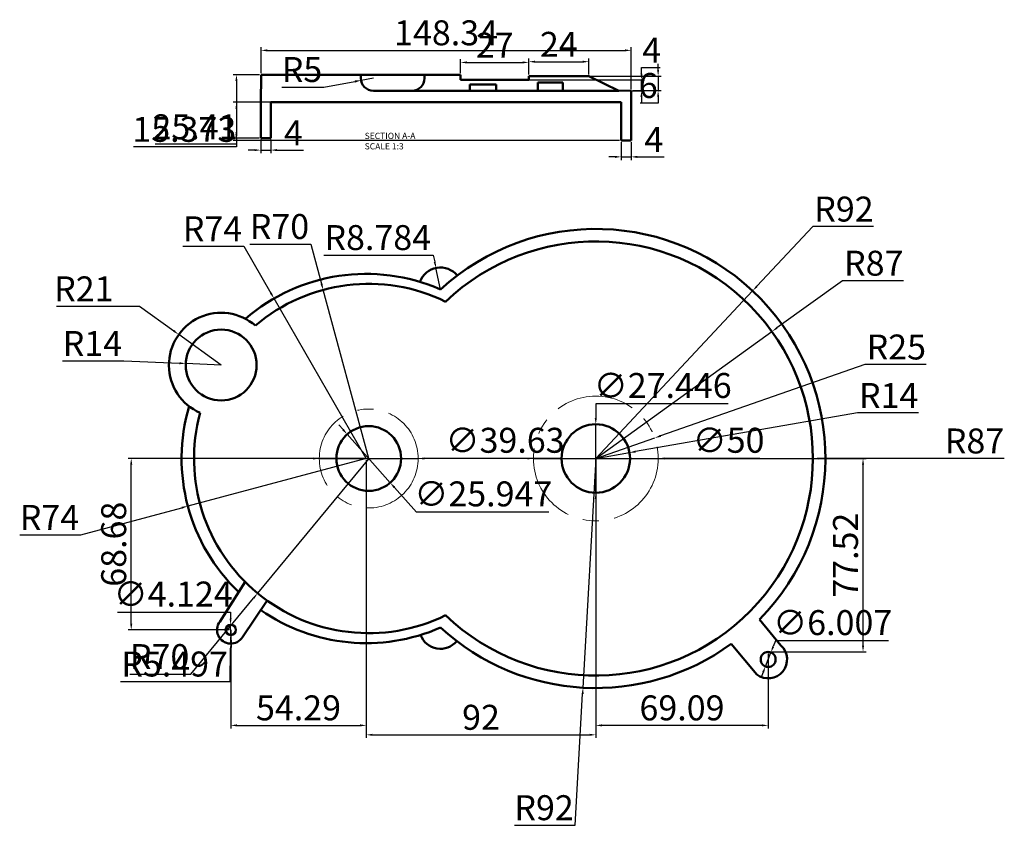
# Model space of a CAD drawing. Units: millimetres. Extents: x 828 to 2987, y 979 to 1807.
# Tile 3 of 6: x 828 to 1223, y 1483 to 1807. Entities that reach past the tile are written whole.
import ezdxf

# ---------------------------------------------------------------- set-up
doc = ezdxf.new("R2010")
doc.units = ezdxf.units.MM
doc.linetypes.add('CENTER', pattern=[50.8, 31.75, -6.35, 6.35, -6.35])
for name, color, linetype, lineweight in [('M-CNTR', 1, 'CENTER', 18), ('M-DIMS', 2, 'Continuous', 25), ('M-OUTL', 7, 'Continuous', 50), ('M-TEXT', 3, 'Continuous', 25)]:
    doc.layers.add(name, color=color, linetype=linetype, lineweight=lineweight)
doc.styles.get("Standard").update_dxf_attribs({"font": 'arial.ttf'})
doc.dimstyles.new('ISO-25', dxfattribs={"dimtxt": 10, "dimasz": 2.5, "dimexe": 1.25, "dimexo": 0.625, "dimtad": 1, "dimtoh": 1, "dimdec": 0, "dimtxsty": 'Standard', "dimcen": 2.5, "dimadec": 0, "dimazin": 0, "dimtfac": 1, "dimtdec": 0, "dimtmove": 0, "dimatfit": 3, "dimfxl": 1, "dimarcsym": 0})

# ---------------------------------------------------------------- blocks, each defined once
blk = doc.blocks.new('*D1')
at = {"layer": 'Defpoints', "color": 0, "transparency": 16777216}
for p in [(1056.44, 1789.71), (1032.41, 1783.89), (1056.44, 1783.91)]:
    blk.add_point(p, dxfattribs=at)
at = {"layer": 'M-DIMS', "color": 0, "lineweight": -2, "transparency": 16777216}
for p, q in [((1032.41, 1784.52), (1032.41, 1790.96)), ((1034.91, 1789.71), (1053.94, 1789.71)), ((1056.44, 1784.53), (1056.44, 1790.96))]:
    blk.add_line(p, q, dxfattribs=at)
at = {"layer": 'M-DIMS', "color": 0, "transparency": 16777216}
for points in [[(1034.91, 1790.13), (1034.91, 1789.29), (1032.41, 1789.71)], [(1053.94, 1790.13), (1053.94, 1789.29), (1056.44, 1789.71)]]:
    blk.add_solid(points, dxfattribs=at)
at = {"layer": 'M-DIMS', "color": 0, "transparency": 16777216, "insert": (1044.43, 1795.36), "char_height": 10, "attachment_point": 5}
blk.add_mtext('24', dxfattribs=at)
blk = doc.blocks.new('*D2')
at = {"layer": 'Defpoints', "color": 0, "transparency": 16777216}
for p in [(1032.41, 1789.42), (1005.08, 1784.49), (1032.41, 1783.89)]:
    blk.add_point(p, dxfattribs=at)
at = {"layer": 'M-DIMS', "color": 0, "lineweight": -2, "transparency": 16777216}
for p, q in [((1005.08, 1785.12), (1005.08, 1790.67)), ((1007.58, 1789.42), (1029.91, 1789.42)), ((1032.41, 1784.52), (1032.41, 1790.67))]:
    blk.add_line(p, q, dxfattribs=at)
at = {"layer": 'M-DIMS', "color": 0, "transparency": 16777216}
for points in [[(1007.58, 1789.83), (1007.58, 1789), (1005.08, 1789.42)], [(1029.91, 1789.83), (1029.91, 1789), (1032.41, 1789.42)]]:
    blk.add_solid(points, dxfattribs=at)
at = {"layer": 'M-DIMS', "color": 0, "transparency": 16777216, "insert": (1018.74, 1795.06), "char_height": 10, "attachment_point": 5}
blk.add_mtext('27', dxfattribs=at)
blk = doc.blocks.new('*D3')
at = {"layer": 'Defpoints', "color": 0, "transparency": 16777216}
for p in [(965.17, 1782.19), (970.09, 1783.06)]:
    blk.add_point(p, dxfattribs=at)
at = {"layer": 'M-DIMS', "color": 0, "lineweight": -2, "transparency": 16777216}
for p, q in [((950.23, 1779.56), (962.7, 1781.76)), ((970.09, 1783.06), (965.17, 1782.19)), ((933.4, 1779.56), (950.23, 1779.56))]:
    blk.add_line(p, q, dxfattribs=at)
at = {"layer": 'M-DIMS', "color": 0, "transparency": 16777216}
blk.add_solid([(962.63, 1782.17), (962.78, 1781.35), (965.17, 1782.19)], dxfattribs=at)
at = {"layer": 'M-DIMS', "color": 0, "transparency": 16777216, "insert": (941.5, 1785.27), "char_height": 10, "attachment_point": 5}
blk.add_mtext('R5', dxfattribs=at)
blk = doc.blocks.new('*D4')
at = {"layer": 'Defpoints', "color": 0, "transparency": 16777216}
for p in [(924.98, 1759.09), (928.98, 1759.09), (928.98, 1754.27)]:
    blk.add_point(p, dxfattribs=at)
at = {"layer": 'M-DIMS', "color": 0, "lineweight": -2, "transparency": 16777216}
for p, q in [((924.98, 1758.46), (924.98, 1753.02)), ((928.98, 1758.46), (928.98, 1753.02)), ((922.48, 1754.27), (919.98, 1754.27)), ((924.98, 1754.27), (928.98, 1754.27)), ((931.48, 1754.27), (942.15, 1754.27))]:
    blk.add_line(p, q, dxfattribs=at)
at = {"layer": 'M-DIMS', "color": 0, "transparency": 16777216}
for points in [[(922.48, 1754.69), (922.48, 1753.86), (924.98, 1754.27)], [(931.48, 1754.69), (931.48, 1753.86), (928.98, 1754.27)]]:
    blk.add_solid(points, dxfattribs=at)
at = {"layer": 'M-DIMS', "color": 0, "transparency": 16777216, "insert": (938.06, 1759.9), "char_height": 10, "attachment_point": 5}
blk.add_mtext('4', dxfattribs=at)
blk = doc.blocks.new('*D5')
at = {"layer": 'Defpoints', "color": 0, "transparency": 16777216}
for p in [(1069.41, 1758.06), (1073.41, 1758.06), (1073.41, 1751.56)]:
    blk.add_point(p, dxfattribs=at)
at = {"layer": 'M-DIMS', "color": 0, "lineweight": -2, "transparency": 16777216}
for p, q in [((1069.41, 1757.44), (1069.41, 1750.31)), ((1073.41, 1757.44), (1073.41, 1750.31)), ((1066.91, 1751.56), (1064.41, 1751.56)), ((1069.41, 1751.56), (1073.41, 1751.56)), ((1075.91, 1751.56), (1086.58, 1751.56))]:
    blk.add_line(p, q, dxfattribs=at)
at = {"layer": 'M-DIMS', "color": 0, "transparency": 16777216}
for points in [[(1066.91, 1751.98), (1066.91, 1751.14), (1069.41, 1751.56)], [(1075.91, 1751.98), (1075.91, 1751.14), (1073.41, 1751.56)]]:
    blk.add_solid(points, dxfattribs=at)
at = {"layer": 'M-DIMS', "color": 0, "transparency": 16777216, "insert": (1082.49, 1757.18), "char_height": 10, "attachment_point": 5}
blk.add_mtext('4', dxfattribs=at)
blk = doc.blocks.new('*D6')
at = {"layer": 'Defpoints', "color": 0, "transparency": 16777216}
for p in [(1056.44, 1783.91), (1073.41, 1778.14), (1084.22, 1778.14)]:
    blk.add_point(p, dxfattribs=at)
at = {"layer": 'M-DIMS', "color": 0, "lineweight": -2, "transparency": 16777216}
for p, q in [((1084.22, 1786.41), (1084.22, 1788.91)), ((1057.07, 1783.91), (1085.47, 1783.91)), ((1084.22, 1783.91), (1084.22, 1778.14)), ((1074.04, 1778.14), (1085.47, 1778.14)), ((1084.22, 1773.14), (1076.99, 1773.14)), ((1084.22, 1775.64), (1084.22, 1773.14))]:
    blk.add_line(p, q, dxfattribs=at)
at = {"layer": 'M-DIMS', "color": 0, "transparency": 16777216}
for points in [[(1083.8, 1786.41), (1084.63, 1786.41), (1084.22, 1783.91)], [(1083.8, 1775.64), (1084.63, 1775.64), (1084.22, 1778.14)]]:
    blk.add_solid(points, dxfattribs=at)
at = {"layer": 'M-DIMS', "color": 0, "transparency": 16777216, "insert": (1080.29, 1778.87), "char_height": 10, "attachment_point": 5}
blk.add_mtext('6', dxfattribs=at)
blk = doc.blocks.new('*D7')
at = {"layer": 'Defpoints', "color": 0, "transparency": 16777216}
for p in [(1018.74, 1782.42), (1077.55, 1782.42), (1019.25, 1778.06)]:
    blk.add_point(p, dxfattribs=at)
at = {"layer": 'M-DIMS', "color": 0, "lineweight": -2, "transparency": 16777216}
for p, q in [((1077.55, 1784.92), (1077.55, 1787.42)), ((1077.55, 1787.42), (1085.09, 1787.42)), ((1019.37, 1782.42), (1078.8, 1782.42)), ((1077.55, 1778.06), (1077.55, 1782.42)), ((1019.88, 1778.06), (1078.8, 1778.06)), ((1077.55, 1775.56), (1077.55, 1773.06))]:
    blk.add_line(p, q, dxfattribs=at)
at = {"layer": 'M-DIMS', "color": 0, "transparency": 16777216}
for points in [[(1077.13, 1784.92), (1077.96, 1784.92), (1077.55, 1782.42)], [(1077.13, 1775.56), (1077.96, 1775.56), (1077.55, 1778.06)]]:
    blk.add_solid(points, dxfattribs=at)
at = {"layer": 'M-DIMS', "color": 0, "transparency": 16777216, "insert": (1081.63, 1793.05), "char_height": 10, "attachment_point": 5}
blk.add_mtext('4', dxfattribs=at)
blk = doc.blocks.new('*D8')
at = {"layer": 'Defpoints', "color": 0, "transparency": 16777216}
for p in [(1122.09, 1697.87), (1059.24, 1630.68)]:
    blk.add_point(p, dxfattribs=at)
at = {"layer": 'M-DIMS', "color": 0, "lineweight": -2, "transparency": 16777216}
for p, q in [((1146.17, 1723.61), (1123.8, 1699.69)), ((1170.59, 1723.61), (1146.17, 1723.61)), ((1059.24, 1630.68), (1122.09, 1697.87))]:
    blk.add_line(p, q, dxfattribs=at)
at = {"layer": 'M-DIMS', "color": 0, "transparency": 16777216}
blk.add_solid([(1123.49, 1699.98), (1124.1, 1699.41), (1122.09, 1697.87)], dxfattribs=at)
at = {"layer": 'M-DIMS', "color": 0, "transparency": 16777216, "insert": (1158.69, 1729.35), "char_height": 10, "attachment_point": 5}
blk.add_mtext('R92', dxfattribs=at)
blk = doc.blocks.new('*D9')
at = {"layer": 'Defpoints', "color": 0, "transparency": 16777216}
for p in [(1129.81, 1681.56), (1059.24, 1630.68)]:
    blk.add_point(p, dxfattribs=at)
at = {"layer": 'M-DIMS', "color": 0, "lineweight": -2, "transparency": 16777216}
for p, q in [((1158.06, 1701.91), (1131.84, 1683.02)), ((1182.58, 1701.91), (1158.06, 1701.91)), ((1059.24, 1630.68), (1129.81, 1681.56))]:
    blk.add_line(p, q, dxfattribs=at)
at = {"layer": 'M-DIMS', "color": 0, "transparency": 16777216}
blk.add_solid([(1131.6, 1683.36), (1132.09, 1682.68), (1129.81, 1681.56)], dxfattribs=at)
at = {"layer": 'M-DIMS', "color": 0, "transparency": 16777216, "insert": (1170.63, 1707.65), "char_height": 10, "attachment_point": 5}
blk.add_mtext('R87', dxfattribs=at)
blk = doc.blocks.new('*D10')
at = {"layer": 'Defpoints', "color": 0, "transparency": 16777216}
for p in [(1082.84, 1638.92), (1059.24, 1630.68)]:
    blk.add_point(p, dxfattribs=at)
at = {"layer": 'M-DIMS', "color": 0, "lineweight": -2, "transparency": 16777216}
for p, q in [((1167.07, 1668.34), (1085.2, 1639.75)), ((1191.67, 1668.34), (1167.07, 1668.34)), ((1059.24, 1630.68), (1082.84, 1638.92))]:
    blk.add_line(p, q, dxfattribs=at)
at = {"layer": 'M-DIMS', "color": 0, "transparency": 16777216}
blk.add_solid([(1085.06, 1640.14), (1085.34, 1639.35), (1082.84, 1638.92)], dxfattribs=at)
at = {"layer": 'M-DIMS', "color": 0, "transparency": 16777216, "insert": (1179.68, 1674.07), "char_height": 10, "attachment_point": 5}
blk.add_mtext('R25', dxfattribs=at)
blk = doc.blocks.new('*D11')
at = {"layer": 'Defpoints', "color": 0, "transparency": 16777216}
for p in [(1059.24, 1630.68), (1072.76, 1633.04)]:
    blk.add_point(p, dxfattribs=at)
at = {"layer": 'M-DIMS', "color": 0, "lineweight": -2, "transparency": 16777216}
for p, q in [((1164.06, 1648.99), (1075.22, 1633.47)), ((1188.54, 1648.99), (1164.06, 1648.99)), ((1059.24, 1630.68), (1072.76, 1633.04))]:
    blk.add_line(p, q, dxfattribs=at)
at = {"layer": 'M-DIMS', "color": 0, "transparency": 16777216}
blk.add_solid([(1075.15, 1633.88), (1075.29, 1633.06), (1072.76, 1633.04)], dxfattribs=at)
at = {"layer": 'M-DIMS', "color": 0, "transparency": 16777216, "insert": (1176.61, 1654.64), "char_height": 10, "attachment_point": 5}
blk.add_mtext('R14', dxfattribs=at)
blk = doc.blocks.new('*D12')
at = {"layer": 'Defpoints', "color": 0, "transparency": 16777216}
for p in [(930.29, 1694.8), (967.24, 1630.68)]:
    blk.add_point(p, dxfattribs=at)
at = {"layer": 'M-DIMS', "color": 0, "lineweight": -2, "transparency": 16777216}
for p, q in [((893.71, 1715.79), (918.19, 1715.79)), ((918.19, 1715.79), (929.04, 1696.96)), ((967.24, 1630.68), (930.29, 1694.8))]:
    blk.add_line(p, q, dxfattribs=at)
at = {"layer": 'M-DIMS', "color": 0, "transparency": 16777216}
blk.add_solid([(929.4, 1697.17), (928.68, 1696.75), (930.29, 1694.8)], dxfattribs=at)
at = {"layer": 'M-DIMS', "color": 0, "transparency": 16777216, "insert": (905.64, 1721.42), "char_height": 10, "attachment_point": 5}
blk.add_mtext('R74', dxfattribs=at)
blk = doc.blocks.new('*D13')
at = {"layer": 'Defpoints', "color": 0, "transparency": 16777216}
for p in [(949.98, 1698.26), (968.24, 1630.68)]:
    blk.add_point(p, dxfattribs=at)
at = {"layer": 'M-DIMS', "color": 0, "lineweight": -2, "transparency": 16777216}
for p, q in [((920.54, 1716.62), (945.03, 1716.62)), ((945.03, 1716.62), (949.33, 1700.67)), ((968.24, 1630.68), (949.98, 1698.26))]:
    blk.add_line(p, q, dxfattribs=at)
at = {"layer": 'M-DIMS', "color": 0, "transparency": 16777216}
blk.add_solid([(949.74, 1700.78), (948.93, 1700.56), (949.98, 1698.26)], dxfattribs=at)
at = {"layer": 'M-DIMS', "color": 0, "transparency": 16777216, "insert": (932.47, 1722.35), "char_height": 10, "attachment_point": 5}
blk.add_mtext('R70', dxfattribs=at)
blk = doc.blocks.new('*D14')
at = {"layer": 'Defpoints', "color": 0, "transparency": 16777216}
for p in [(892.12, 1680.39), (909.1, 1668.14)]:
    blk.add_point(p, dxfattribs=at)
at = {"layer": 'M-DIMS', "color": 0, "lineweight": -2, "transparency": 16777216}
for p, q in [((843.09, 1691.73), (876.39, 1691.73)), ((876.39, 1691.73), (890.09, 1681.85)), ((909.1, 1668.14), (892.12, 1680.39))]:
    blk.add_line(p, q, dxfattribs=at)
at = {"layer": 'M-DIMS', "color": 0, "transparency": 16777216}
blk.add_solid([(890.33, 1682.19), (889.84, 1681.51), (892.12, 1680.39)], dxfattribs=at)
at = {"layer": 'M-DIMS', "color": 0, "transparency": 16777216, "insert": (854.07, 1697.37), "char_height": 10, "attachment_point": 5}
blk.add_mtext('R21', dxfattribs=at)
blk = doc.blocks.new('*D15')
at = {"layer": 'Defpoints', "color": 0, "transparency": 16777216}
for p in [(894.91, 1668.76), (909.1, 1668.14)]:
    blk.add_point(p, dxfattribs=at)
at = {"layer": 'M-DIMS', "color": 0, "lineweight": -2, "transparency": 16777216}
for p, q in [((845.58, 1669.84), (870.06, 1669.84)), ((870.06, 1669.84), (892.41, 1668.87)), ((909.1, 1668.14), (894.91, 1668.76))]:
    blk.add_line(p, q, dxfattribs=at)
at = {"layer": 'M-DIMS', "color": 0, "transparency": 16777216}
blk.add_solid([(892.43, 1669.28), (892.39, 1668.45), (894.91, 1668.76)], dxfattribs=at)
at = {"layer": 'M-DIMS', "color": 0, "transparency": 16777216, "insert": (857.51, 1675.49), "char_height": 10, "attachment_point": 5}
blk.add_mtext('R14', dxfattribs=at)
blk = doc.blocks.new('*D16')
at = {"layer": 'Defpoints', "color": 0, "transparency": 16777216}
for p in [(967.24, 1630.68), (1059.24, 1630.68), (1059.24, 1519.94)]:
    blk.add_point(p, dxfattribs=at)
at = {"layer": 'M-DIMS', "color": 0, "lineweight": -2, "transparency": 16777216}
for p, q in [((967.24, 1630.06), (967.24, 1518.69)), ((1059.24, 1630.06), (1059.24, 1518.69)), ((969.74, 1519.94), (1056.74, 1519.94))]:
    blk.add_line(p, q, dxfattribs=at)
at = {"layer": 'M-DIMS', "color": 0, "transparency": 16777216}
for points in [[(969.74, 1520.36), (969.74, 1519.53), (967.24, 1519.94)], [(1056.74, 1520.36), (1056.74, 1519.53), (1059.24, 1519.94)]]:
    blk.add_solid(points, dxfattribs=at)
at = {"layer": 'M-DIMS', "color": 0, "transparency": 16777216, "insert": (1013.24, 1525.67), "char_height": 10, "attachment_point": 5}
blk.add_mtext('92', dxfattribs=at)
blk = doc.blocks.new('*D70')
at = {"layer": 'Defpoints', "color": 0, "transparency": 16777216}
for p in [(967.24, 1630.68), (912.95, 1562), (967.24, 1523.72)]:
    blk.add_point(p, dxfattribs=at)
at = {"layer": 'M-DIMS', "color": 0, "lineweight": -2, "transparency": 16777216}
for p, q in [((967.24, 1630.06), (967.24, 1522.47)), ((912.95, 1561.37), (912.95, 1522.47)), ((915.45, 1523.72), (964.74, 1523.72))]:
    blk.add_line(p, q, dxfattribs=at)
at = {"layer": 'M-DIMS', "color": 0, "transparency": 16777216}
for points in [[(915.45, 1524.14), (915.45, 1523.31), (912.95, 1523.72)], [(964.74, 1524.14), (964.74, 1523.31), (967.24, 1523.72)]]:
    blk.add_solid(points, dxfattribs=at)
at = {"layer": 'M-DIMS', "color": 0, "transparency": 16777216, "insert": (940.1, 1529.45), "char_height": 10, "attachment_point": 5}
blk.add_mtext('54.29', dxfattribs=at)
blk = doc.blocks.new('*D71')
at = {"layer": 'Defpoints', "color": 0, "transparency": 16777216}
for p in [(873.06, 1630.68), (967.24, 1630.68), (912.95, 1562)]:
    blk.add_point(p, dxfattribs=at)
at = {"layer": 'M-DIMS', "color": 0, "lineweight": -2, "transparency": 16777216}
for p, q in [((966.61, 1630.68), (871.81, 1630.68)), ((873.06, 1564.5), (873.06, 1628.18)), ((912.33, 1562), (871.81, 1562))]:
    blk.add_line(p, q, dxfattribs=at)
at = {"layer": 'M-DIMS', "color": 0, "transparency": 16777216}
for points in [[(872.64, 1628.18), (873.48, 1628.18), (873.06, 1630.68)], [(872.64, 1564.5), (873.48, 1564.5), (873.06, 1562)]]:
    blk.add_solid(points, dxfattribs=at)
at = {"layer": 'M-DIMS', "color": 0, "transparency": 16777216, "insert": (867.33, 1596.34), "char_height": 10, "attachment_point": 5, "rotation": 90}
blk.add_mtext('68.68', dxfattribs=at)
blk = doc.blocks.new('*D72')
at = {"layer": 'Defpoints', "color": 0, "transparency": 16777216}
for p in [(1059.24, 1630.68), (1128.32, 1553.16), (1059.24, 1523.72)]:
    blk.add_point(p, dxfattribs=at)
at = {"layer": 'M-DIMS', "color": 0, "lineweight": -2, "transparency": 16777216}
for p, q in [((1059.24, 1630.06), (1059.24, 1522.47)), ((1128.32, 1552.53), (1128.32, 1522.47)), ((1125.82, 1523.72), (1061.74, 1523.72))]:
    blk.add_line(p, q, dxfattribs=at)
at = {"layer": 'M-DIMS', "color": 0, "transparency": 16777216}
for points in [[(1061.74, 1524.14), (1061.74, 1523.31), (1059.24, 1523.72)], [(1125.82, 1524.14), (1125.82, 1523.31), (1128.32, 1523.72)]]:
    blk.add_solid(points, dxfattribs=at)
at = {"layer": 'M-DIMS', "color": 0, "transparency": 16777216, "insert": (1093.78, 1529.45), "char_height": 10, "attachment_point": 5}
blk.add_mtext('69.09', dxfattribs=at)
blk = doc.blocks.new('*D73')
at = {"layer": 'Defpoints', "color": 0, "transparency": 16777216}
for p in [(1059.24, 1630.68), (1166.34, 1630.68), (1128.32, 1553.16)]:
    blk.add_point(p, dxfattribs=at)
at = {"layer": 'M-DIMS', "color": 0, "lineweight": -2, "transparency": 16777216}
for p, q in [((1059.86, 1630.68), (1167.59, 1630.68)), ((1166.34, 1555.66), (1166.34, 1628.18)), ((1128.95, 1553.16), (1167.59, 1553.16))]:
    blk.add_line(p, q, dxfattribs=at)
at = {"layer": 'M-DIMS', "color": 0, "transparency": 16777216}
for points in [[(1165.92, 1628.18), (1166.76, 1628.18), (1166.34, 1630.68)], [(1165.92, 1555.66), (1166.76, 1555.66), (1166.34, 1553.16)]]:
    blk.add_solid(points, dxfattribs=at)
at = {"layer": 'M-DIMS', "color": 0, "transparency": 16777216, "insert": (1160.61, 1591.92), "char_height": 10, "attachment_point": 5, "rotation": 90}
blk.add_mtext('77.52', dxfattribs=at)
blk = doc.blocks.new('*D74')
at = {"layer": 'Defpoints', "color": 0, "transparency": 16777216}
for p in [(1073.41, 1794.24), (925.07, 1784.49), (1073.41, 1778.14)]:
    blk.add_point(p, dxfattribs=at)
at = {"layer": 'M-DIMS', "color": 0, "lineweight": -2, "transparency": 16777216}
for p, q in [((925.07, 1785.12), (925.07, 1795.49)), ((1073.41, 1778.76), (1073.41, 1795.49)), ((927.57, 1794.24), (1070.91, 1794.24))]:
    blk.add_line(p, q, dxfattribs=at)
at = {"layer": 'M-DIMS', "color": 0, "transparency": 16777216}
for points in [[(927.57, 1794.66), (927.57, 1793.83), (925.07, 1794.24)], [(1070.91, 1794.66), (1070.91, 1793.83), (1073.41, 1794.24)]]:
    blk.add_solid(points, dxfattribs=at)
at = {"layer": 'M-DIMS', "color": 0, "transparency": 16777216, "insert": (999.24, 1799.98), "char_height": 10, "attachment_point": 5}
blk.add_mtext('148.34', dxfattribs=at)
blk = doc.blocks.new('*D75')
at = {"layer": 'Defpoints', "color": 0, "transparency": 16777216}
for p in [(925.07, 1784.49), (915.23, 1759.09), (924.98, 1759.09)]:
    blk.add_point(p, dxfattribs=at)
at = {"layer": 'M-DIMS', "color": 0, "lineweight": -2, "transparency": 16777216}
for p, q in [((924.45, 1784.49), (913.98, 1784.49)), ((915.23, 1781.99), (915.23, 1761.59)), ((915.23, 1756.59), (882.62, 1756.59)), ((924.35, 1759.09), (913.98, 1759.09)), ((915.23, 1759.09), (915.23, 1756.59))]:
    blk.add_line(p, q, dxfattribs=at)
at = {"layer": 'M-DIMS', "color": 0, "transparency": 16777216}
for points in [[(914.81, 1781.99), (915.65, 1781.99), (915.23, 1784.49)], [(914.81, 1761.59), (915.65, 1761.59), (915.23, 1759.09)]]:
    blk.add_solid(points, dxfattribs=at)
at = {"layer": 'M-DIMS', "color": 0, "transparency": 16777216, "insert": (898.61, 1762.32), "char_height": 10, "attachment_point": 5}
blk.add_mtext('25.41', dxfattribs=at)
blk = doc.blocks.new('*D76')
at = {"layer": 'Defpoints', "color": 0, "transparency": 16777216}
for p in [(1069.41, 1773.44), (915.23, 1758.06), (1069.41, 1758.06)]:
    blk.add_point(p, dxfattribs=at)
at = {"layer": 'M-DIMS', "color": 0, "lineweight": -2, "transparency": 16777216}
for p, q in [((1068.79, 1773.44), (913.98, 1773.44)), ((915.23, 1770.94), (915.23, 1760.56)), ((1068.79, 1758.06), (913.98, 1758.06)), ((915.23, 1758.06), (915.23, 1755.56)), ((915.23, 1755.56), (874.03, 1755.56))]:
    blk.add_line(p, q, dxfattribs=at)
at = {"layer": 'M-DIMS', "color": 0, "transparency": 16777216}
for points in [[(914.81, 1770.94), (915.65, 1770.94), (915.23, 1773.44)], [(914.81, 1760.56), (915.65, 1760.56), (915.23, 1758.06)]]:
    blk.add_solid(points, dxfattribs=at)
at = {"layer": 'M-DIMS', "color": 0, "transparency": 16777216, "insert": (894.32, 1761.3), "char_height": 10, "attachment_point": 5}
blk.add_mtext('15.373', dxfattribs=at)
blk = doc.blocks.new('*D112')
at = {"layer": 'Defpoints', "color": 0, "transparency": 16777216}
for p in [(1059.24, 1630.68), (1054.11, 1538.82)]:
    blk.add_point(p, dxfattribs=at)
at = {"layer": 'M-DIMS', "color": 0, "lineweight": -2, "transparency": 16777216}
for p, q in [((1059.24, 1630.68), (1054.11, 1538.82)), ((1051.03, 1483.71), (1053.97, 1536.33)), ((1026.62, 1483.71), (1051.03, 1483.71))]:
    blk.add_line(p, q, dxfattribs=at)
at = {"layer": 'M-DIMS', "color": 0, "transparency": 16777216}
blk.add_solid([(1053.56, 1536.35), (1054.39, 1536.3), (1054.11, 1538.82)], dxfattribs=at)
at = {"layer": 'M-DIMS', "color": 0, "transparency": 16777216, "insert": (1038.51, 1489.44), "char_height": 10, "attachment_point": 5}
blk.add_mtext('R92', dxfattribs=at)
blk = doc.blocks.new('*D113')
at = {"layer": 'Defpoints', "color": 0, "transparency": 16777216}
for p in [(1059.24, 1630.68), (1146.24, 1630.68)]:
    blk.add_point(p, dxfattribs=at)
at = {"layer": 'M-DIMS', "color": 0, "lineweight": -2, "transparency": 16777216}
for p, q in [((1059.24, 1630.68), (1146.24, 1630.68)), ((1198.44, 1630.68), (1148.74, 1630.68)), ((1222.96, 1630.68), (1198.44, 1630.68))]:
    blk.add_line(p, q, dxfattribs=at)
at = {"layer": 'M-DIMS', "color": 0, "transparency": 16777216}
blk.add_solid([(1148.74, 1631.1), (1148.74, 1630.26), (1146.24, 1630.68)], dxfattribs=at)
at = {"layer": 'M-DIMS', "color": 0, "transparency": 16777216, "insert": (1211.01, 1636.41), "char_height": 10, "attachment_point": 5}
blk.add_mtext('R87', dxfattribs=at)
blk = doc.blocks.new('*D114')
at = {"layer": 'Defpoints', "color": 0, "transparency": 16777216}
for p in [(967.24, 1630.68), (895.74, 1611.6)]:
    blk.add_point(p, dxfattribs=at)
at = {"layer": 'M-DIMS', "color": 0, "lineweight": -2, "transparency": 16777216}
for p, q in [((967.24, 1630.68), (895.74, 1611.6)), ((852.84, 1600.15), (893.33, 1610.96)), ((828.36, 1600.15), (852.84, 1600.15))]:
    blk.add_line(p, q, dxfattribs=at)
at = {"layer": 'M-DIMS', "color": 0, "transparency": 16777216}
blk.add_solid([(893.22, 1611.36), (893.43, 1610.55), (895.74, 1611.6)], dxfattribs=at)
at = {"layer": 'M-DIMS', "color": 0, "transparency": 16777216, "insert": (840.29, 1605.78), "char_height": 10, "attachment_point": 5}
blk.add_mtext('R74', dxfattribs=at)
blk = doc.blocks.new('*D115')
at = {"layer": 'Defpoints', "color": 0, "transparency": 16777216}
for p in [(968.24, 1630.68), (923.71, 1576.67)]:
    blk.add_point(p, dxfattribs=at)
at = {"layer": 'M-DIMS', "color": 0, "lineweight": -2, "transparency": 16777216}
for p, q in [((968.24, 1630.68), (923.71, 1576.67)), ((896.99, 1544.26), (922.12, 1574.74)), ((872.51, 1544.26), (896.99, 1544.26))]:
    blk.add_line(p, q, dxfattribs=at)
at = {"layer": 'M-DIMS', "color": 0, "transparency": 16777216}
blk.add_solid([(921.8, 1575.01), (922.44, 1574.48), (923.71, 1576.67)], dxfattribs=at)
at = {"layer": 'M-DIMS', "color": 0, "transparency": 16777216, "insert": (884.44, 1549.99), "char_height": 10, "attachment_point": 5}
blk.add_mtext('R70', dxfattribs=at)
blk = doc.blocks.new('*D116')
at = {"layer": 'Defpoints', "color": 0, "transparency": 16777216}
for p in [(1034.24, 1630.68), (1084.24, 1630.68)]:
    blk.add_point(p, dxfattribs=at)
at = {"layer": 'M-DIMS', "color": 0, "lineweight": -2, "transparency": 16777216}
for p, q in [((1031.74, 1630.68), (1029.24, 1630.68)), ((1034.24, 1630.68), (1084.24, 1630.68)), ((1099.24, 1630.68), (1086.74, 1630.68)), ((1125.03, 1630.68), (1099.24, 1630.68))]:
    blk.add_line(p, q, dxfattribs=at)
at = {"layer": 'M-DIMS', "color": 0, "transparency": 16777216}
for points in [[(1031.74, 1631.1), (1031.74, 1630.26), (1034.24, 1630.68)], [(1086.74, 1631.1), (1086.74, 1630.26), (1084.24, 1630.68)]]:
    blk.add_solid(points, dxfattribs=at)
at = {"layer": 'M-DIMS', "color": 0, "transparency": 16777216, "insert": (1112.45, 1636.69), "char_height": 10, "attachment_point": 5}
blk.add_mtext('∅50', dxfattribs=at)
blk = doc.blocks.new('*D117')
at = {"layer": 'Defpoints', "color": 0, "transparency": 16777216}
for p in [(948.43, 1630.68), (988.05, 1630.68)]:
    blk.add_point(p, dxfattribs=at)
at = {"layer": 'M-DIMS', "color": 0, "lineweight": -2, "transparency": 16777216}
for p, q in [((945.93, 1630.68), (943.43, 1630.68)), ((948.43, 1630.68), (988.05, 1630.68)), ((999.94, 1630.68), (990.55, 1630.68)), ((1045.19, 1630.68), (999.94, 1630.68))]:
    blk.add_line(p, q, dxfattribs=at)
at = {"layer": 'M-DIMS', "color": 0, "transparency": 16777216}
for points in [[(945.93, 1631.1), (945.93, 1630.26), (948.43, 1630.68)], [(990.55, 1631.1), (990.55, 1630.26), (988.05, 1630.68)]]:
    blk.add_solid(points, dxfattribs=at)
at = {"layer": 'M-DIMS', "color": 0, "transparency": 16777216, "insert": (1022.88, 1636.69), "char_height": 10, "attachment_point": 5}
blk.add_mtext('∅39.63', dxfattribs=at)
blk = doc.blocks.new('*D118')
at = {"layer": 'Defpoints', "color": 0, "transparency": 16777216}
for p in [(1059.24, 1644.4), (1059.24, 1616.96)]:
    blk.add_point(p, dxfattribs=at)
at = {"layer": 'M-DIMS', "color": 0, "lineweight": -2, "transparency": 16777216}
for p, q in [((1112.25, 1652.64), (1059.24, 1652.64)), ((1059.24, 1652.64), (1059.24, 1646.9)), ((1059.24, 1616.96), (1059.24, 1644.4)), ((1059.24, 1614.46), (1059.24, 1611.96))]:
    blk.add_line(p, q, dxfattribs=at)
at = {"layer": 'M-DIMS', "color": 0, "transparency": 16777216}
for points in [[(1058.82, 1646.9), (1059.66, 1646.9), (1059.24, 1644.4)], [(1058.82, 1614.46), (1059.65, 1614.46), (1059.24, 1616.96)]]:
    blk.add_solid(points, dxfattribs=at)
at = {"layer": 'M-DIMS', "color": 0, "transparency": 16777216, "insert": (1086.06, 1658.65), "char_height": 10, "attachment_point": 5}
blk.add_mtext('∅27.446', dxfattribs=at)
blk = doc.blocks.new('*D119')
at = {"layer": 'Defpoints', "color": 0, "transparency": 16777216}
for p in [(959.62, 1640.38), (976.86, 1620.98)]:
    blk.add_point(p, dxfattribs=at)
at = {"layer": 'M-DIMS', "color": 0, "lineweight": -2, "transparency": 16777216}
for p, q in [((957.96, 1642.25), (956.3, 1644.11)), ((959.62, 1640.38), (976.86, 1620.98)), ((987.34, 1609.2), (978.52, 1619.12)), ((1040.36, 1609.2), (987.34, 1609.2))]:
    blk.add_line(p, q, dxfattribs=at)
at = {"layer": 'M-DIMS', "color": 0, "transparency": 16777216}
for points in [[(958.27, 1642.52), (957.65, 1641.97), (959.62, 1640.38)], [(978.83, 1619.39), (978.21, 1618.84), (976.86, 1620.98)]]:
    blk.add_solid(points, dxfattribs=at)
at = {"layer": 'M-DIMS', "color": 0, "transparency": 16777216, "insert": (1014.16, 1615.21), "char_height": 10, "attachment_point": 5}
blk.add_mtext('∅25.947', dxfattribs=at)
blk = doc.blocks.new('*D120')
at = {"layer": 'Defpoints', "color": 0, "transparency": 16777216}
for p in [(912.91, 1564.06), (913, 1559.94)]:
    blk.add_point(p, dxfattribs=at)
at = {"layer": 'M-DIMS', "color": 0, "lineweight": -2, "transparency": 16777216}
for p, q in [((867.59, 1569.06), (912.8, 1569.06)), ((912.8, 1569.06), (912.85, 1566.56)), ((913, 1559.94), (912.91, 1564.06)), ((913.05, 1557.44), (913.11, 1554.94))]:
    blk.add_line(p, q, dxfattribs=at)
at = {"layer": 'M-DIMS', "color": 0, "transparency": 16777216}
for points in [[(913.27, 1566.57), (912.43, 1566.55), (912.91, 1564.06)], [(913.47, 1557.45), (912.64, 1557.43), (913, 1559.94)]]:
    blk.add_solid(points, dxfattribs=at)
at = {"layer": 'M-DIMS', "color": 0, "transparency": 16777216, "insert": (889.88, 1575.07), "char_height": 10, "attachment_point": 5}
blk.add_mtext('∅4.124', dxfattribs=at)
blk = doc.blocks.new('*D121')
at = {"layer": 'Defpoints', "color": 0, "transparency": 16777216}
for p in [(912.95, 1562), (912.9, 1556.5)]:
    blk.add_point(p, dxfattribs=at)
at = {"layer": 'M-DIMS', "color": 0, "lineweight": -2, "transparency": 16777216}
for p, q in [((912.95, 1562), (912.9, 1556.5)), ((912.74, 1541.29), (912.87, 1554)), ((868.8, 1541.29), (912.74, 1541.29))]:
    blk.add_line(p, q, dxfattribs=at)
at = {"layer": 'M-DIMS', "color": 0, "transparency": 16777216}
blk.add_solid([(912.46, 1554.01), (913.29, 1554), (912.9, 1556.5)], dxfattribs=at)
at = {"layer": 'M-DIMS', "color": 0, "transparency": 16777216, "insert": (890.46, 1547.02), "char_height": 10, "attachment_point": 5}
blk.add_mtext('R5.497', dxfattribs=at)
blk = doc.blocks.new('*D122')
at = {"layer": 'Defpoints', "color": 0, "transparency": 16777216}
for p in [(1129.42, 1552.95), (1127.23, 1547.36)]:
    blk.add_point(p, dxfattribs=at)
at = {"layer": 'M-DIMS', "color": 0, "lineweight": -2, "transparency": 16777216}
for p, q in [((1131.24, 1557.61), (1130.33, 1555.28)), ((1176.49, 1557.61), (1131.24, 1557.61)), ((1127.23, 1547.36), (1129.42, 1552.95)), ((1126.32, 1545.03), (1125.41, 1542.7))]:
    blk.add_line(p, q, dxfattribs=at)
at = {"layer": 'M-DIMS', "color": 0, "transparency": 16777216}
for points in [[(1129.94, 1555.43), (1130.72, 1555.13), (1129.42, 1552.95)], [(1125.93, 1545.18), (1126.71, 1544.88), (1127.23, 1547.36)]]:
    blk.add_solid(points, dxfattribs=at)
at = {"layer": 'M-DIMS', "color": 0, "transparency": 16777216, "insert": (1154.18, 1563.62), "char_height": 10, "attachment_point": 5}
blk.add_mtext('∅6.007', dxfattribs=at)
blk = doc.blocks.new('*D123')
at = {"layer": 'Defpoints', "color": 0, "transparency": 16777216}
for p in [(995.2, 1707.03), (997, 1698.43)]:
    blk.add_point(p, dxfattribs=at)
at = {"layer": 'M-DIMS', "color": 0, "lineweight": -2, "transparency": 16777216}
for p, q in [((950.23, 1712.19), (994.12, 1712.19)), ((994.12, 1712.19), (994.69, 1709.48)), ((997, 1698.43), (995.2, 1707.03))]:
    blk.add_line(p, q, dxfattribs=at)
at = {"layer": 'M-DIMS', "color": 0, "transparency": 16777216}
blk.add_solid([(995.1, 1709.56), (994.28, 1709.39), (995.2, 1707.03)], dxfattribs=at)
at = {"layer": 'M-DIMS', "color": 0, "transparency": 16777216, "insert": (971.86, 1717.92), "char_height": 10, "attachment_point": 5}
blk.add_mtext('R8.784', dxfattribs=at)

msp = doc.modelspace()

# ---------------------------------------------------------------- linework, layer by layer
at = {"layer": 'M-CNTR'}
msp.add_line((968.2392, 1630.6807), (1059.2392, 1630.6807), dxfattribs=at)
for centre, radius in [((1059.2392, 1630.6807), 25), ((968.2392, 1630.6807), 19.8136)]:
    msp.add_circle(centre, radius, dxfattribs=at)
at = {"layer": 'M-OUTL'}
for p, q in [((925.0723, 1784.4945), (924.9796, 1773.0617)), ((965.0894, 1784.4945), (925.0723, 1784.4945)), ((965.0894, 1783.0617), (965.0894, 1784.4945)), ((965.0894, 1784.4945), (990.591, 1784.4945)), ((990.591, 1784.4945), (990.591, 1783.0617)), ((990.591, 1784.4945), (1005.0775, 1784.4945)), ((1005.0775, 1784.4945), (1005.0775, 1782.4222)), ((1032.4099, 1783.8928), (1035.0734, 1783.91)), ((1032.4099, 1782.4222), (1032.4099, 1783.8928)), ((1035.0734, 1783.91), (1056.4449, 1783.91)), ((1068.4109, 1778.0617), (1056.4449, 1783.91)), ((1005.0775, 1782.4222), (1032.4099, 1782.4222)), ((1019.2501, 1780.5436), (1008.7736, 1780.5436)), ((1008.7736, 1780.5436), (1008.7736, 1778.0617)), ((1019.2501, 1778.0617), (1019.2501, 1780.5436)), ((1036.058, 1778.0617), (1036.058, 1781.4047)), ((1036.058, 1781.4047), (1046.0933, 1781.4047)), ((1046.0933, 1781.4047), (1046.0933, 1778.0617)), ((985.591, 1778.0617), (970.0894, 1778.0617)), ((970.0894, 1778.0617), (1068.4109, 1778.0617)), ((1073.4109, 1778.139), (1068.4109, 1778.0617)), ((1073.4109, 1773.0617), (1073.4109, 1778.139)), ((924.9796, 1773.0617), (924.9796, 1772.0617)), ((924.9796, 1772.0617), (924.9796, 1759.0866)), ((928.9796, 1759.0866), (928.9796, 1773.4351)), ((929.6983, 1773.4351), (928.9796, 1773.4351)), ((929.6983, 1773.4351), (1069.4109, 1773.4351)), ((1069.4109, 1773.4351), (1069.4109, 1758.0617)), ((1073.4109, 1758.0617), (1073.4109, 1773.0617)), ((924.9796, 1759.0866), (928.9796, 1759.0866)), ((1069.4109, 1758.0617), (1073.4109, 1758.0617)), ((908.5315, 1565.2663), (918.689, 1581.2359)), ((917.6286, 1559.1084), (927.5075, 1573.7515)), ((1133.4123, 1555.7729), (1124.8845, 1566.2237)), ((1123.7602, 1544.1065), (1113.5501, 1556.4221))]:
    msp.add_line(p, q, dxfattribs=at)
for centre, radius in [((909.1033, 1668.1366), 14.2063), ((968.2392, 1630.6807), 12.9735), ((1059.2392, 1630.6807), 13.7228), ((912.9522, 1561.9985), 2.0622), ((1128.3242, 1550.1565), 3.0033)]:
    msp.add_circle(centre, radius, dxfattribs=at)
for centre, radius, start, end in [((970.0894, 1783.0617), 5, 180, 270), ((985.591, 1783.0617), 5, 270, 0), ((929.9796, 1773.0617), 5, 179.07074, 180), ((1059.2392, 1630.6807), 92, 315.523323, 132.571698), ((1059.2392, 1630.6807), 87, 226.247083, 133.752917), ((967.2392, 1630.6807), 74, 66.285849, 130.830663), ((997.0001, 1698.4323), 8.7838, 39.835463, 159.688362), ((968.2392, 1630.6807), 70, 63.864062, 130.442012), ((909.1033, 1668.1366), 20.945, 49.046192, 246.254552), ((909.1033, 1668.1366), 20.945, 49.046192, 246.254552), ((967.2392, 1630.6807), 74, 163.583453, 226.297356), ((968.2392, 1630.6807), 70, 164.858732, 296.135938), ((967.2392, 1630.6807), 74, 235.144319, 293.714151), ((912.9522, 1561.9985), 5.4974, 143.528456, 328.283251), ((1059.2392, 1630.6807), 92, 227.428302, 306.180833), ((997.0001, 1562.929), 8.4967, 200.422982, 320.075032), ((1128.3242, 1550.1565), 7.5784, 232.969948, 47.825542)]:
    msp.add_arc(centre, radius, start, end, dxfattribs=at)

# ---------------------------------------------------------------- texts
at = {"layer": 'M-TEXT', "insert": (966.6125, 1761.2204), "char_height": 2.5, "attachment_point": 1}
msp.add_mtext_dynamic_manual_height_columns('SECTION A-A\\PSCALE 1:3', width=74.519771, gutter_width=12.5, heights=[0], dxfattribs=at)

# ---------------------------------------------------------------- dimensions: what is measured, and where the dimension line sits
at = {"layer": 'M-DIMS'}
for base, p1, p2, override, picture, middle in [((1073.4109, 1794.2445), (925.0723, 1784.4945), (1073.4109, 1778.139), {"dimdec": 2, "dimlfac": 1, "dimrnd": 0, "dimzin": 0, "dimdsep": 46, "dimlunit": 2}, '*D74', (999.2416, 1799.9786)), ((1032.4099, 1789.4182), (1005.0775, 1784.4945), (1032.4099, 1783.8928), {"dimclrd": 0, "dimclre": 0, "dimclrt": 0}, '*D2', (1018.7437, 1795.0637)), ((1056.4449, 1789.7105), (1032.4099, 1783.8928), (1056.4449, 1783.91), {"dimclrd": 0, "dimclre": 0, "dimclrt": 0}, '*D1', (1044.4274, 1795.3559)), ((928.9796, 1754.2728), (924.9796, 1759.0866), (928.9796, 1759.0866), {"dimclrd": 0, "dimclre": 0, "dimclrt": 0}, '*D4', (938.063, 1759.8978)), ((1073.4109, 1751.559), (1069.4109, 1758.0617), (1073.4109, 1758.0617), {"dimclrd": 0, "dimclre": 0, "dimclrt": 0}, '*D5', (1082.4943, 1757.184)), ((967.2392, 1523.7237), (912.9522, 1561.9985), (967.2392, 1630.6807), {"dimdec": 2, "dimlfac": 1, "dimrnd": 0, "dimzin": 0, "dimdsep": 46, "dimlunit": 2}, '*D70', (940.0957, 1529.4544)), ((1059.2392, 1519.9427), (967.2392, 1630.6807), (1059.2392, 1630.6807), {"dimclrd": 0, "dimclre": 0, "dimclrt": 0}, '*D16', (1013.2392, 1525.6734)), ((1059.2392, 1523.7237), (1128.32422, 1553.15975), (1059.2392, 1630.68066), {"dimdec": 2, "dimlfac": 1, "dimrnd": 0, "dimzin": 0, "dimdsep": 46, "dimlunit": 2}, '*D72', (1093.78171, 1529.45443))]:
    dim = msp.add_linear_dim(base=base, p1=p1, p2=p2, dimstyle='ISO-25', override=override, dxfattribs=at)
    dim.commit()
    dim.dimension.update_dxf_attribs({"geometry": picture, "text_midpoint": middle})
for base, p1, p2, override, picture, middle in [((1077.5455, 1782.4222), (1019.2501, 1778.0617), (1018.7437, 1782.4222), {"dimclrd": 0, "dimclre": 0, "dimclrt": 0}, '*D7', (1081.6289, 1793.0472)), ((1084.2153, 1778.139), (1056.4449, 1783.91), (1073.4109, 1778.139), {"dimclrd": 0, "dimclre": 0, "dimclrt": 0}, '*D6', (1080.2888, 1778.8697)), ((915.2296, 1759.0866), (925.0723, 1784.4945), (924.9796, 1759.0866), {"dimdec": 2, "dimlfac": 1, "dimrnd": 0, "dimzin": 0, "dimdsep": 46, "dimlunit": 2}, '*D75', (898.6121, 1762.3173)), ((915.2296, 1758.0617), (1069.4109, 1773.4351), (1069.4109, 1758.0617), {"dimdec": 3, "dimlfac": 1, "dimrnd": 0, "dimzin": 0, "dimdsep": 46, "dimlunit": 2}, '*D76', (894.3181, 1761.2958)), ((873.0591, 1630.6807), (912.9522, 1561.9985), (967.2392, 1630.6807), {"dimdec": 2, "dimlfac": 1, "dimrnd": 0, "dimzin": 0, "dimdsep": 46, "dimlunit": 2}, '*D71', (867.3284, 1596.3396)), ((1166.3386, 1630.6807), (1128.3242, 1553.1598), (1059.2392, 1630.6807), {"dimdec": 2, "dimlfac": 1, "dimrnd": 0, "dimzin": 0, "dimdsep": 46, "dimlunit": 2}, '*D73', (1160.6078, 1591.9202))]:
    dim = msp.add_linear_dim(base=base, p1=p1, p2=p2, angle=90, dimstyle='ISO-25', override=override, dxfattribs=at)
    dim.commit()
    dim.dimension.update_dxf_attribs({"geometry": picture, "text_midpoint": middle})
for center, mpoint, override, picture, middle in [((970.0894, 1783.0617), (965.1654, 1782.1931), {"dimclrd": 0, "dimclre": 0, "dimclrt": 0}, '*D3', (941.5002, 1785.2682)), ((912.9522, 1561.9985), (912.897, 1556.5014), {"dimdec": 3, "dimlfac": 1, "dimrnd": 0, "dimzin": 0, "dimdsep": 46, "dimlunit": 2}, '*D121', (890.4616, 1547.0215))]:
    dim = msp.add_radius_dim(center=center, mpoint=mpoint, dimstyle='ISO-25', override=override, dxfattribs=at)
    dim.commit()
    dim.dimension.update_dxf_attribs({"geometry": picture, "text_midpoint": middle})
for center, mpoint, override, picture, middle in [((1059.2392, 1630.6807), (1122.0879, 1697.8673), {"dimclrd": 0, "dimclre": 0, "dimclrt": 0}, '*D8', (1158.6943, 1723.6148)), ((968.2392, 1630.6807), (949.9848, 1698.2586), {"dimclrd": 0, "dimclre": 0, "dimclrt": 0}, '*D13', (932.4703, 1716.6174)), ((967.2392, 1630.6807), (930.2902, 1694.7959), {"dimclrd": 0, "dimclre": 0, "dimclrt": 0}, '*D12', (905.6381, 1715.7924)), ((997.0001, 1698.4323), (995.2027, 1707.0303), {"dimdec": 3, "dimlfac": 1, "dimrnd": 0, "dimzin": 0, "dimdsep": 46, "dimlunit": 2}, '*D123', (971.8622, 1712.1891)), ((1059.2392, 1630.6807), (1129.8139, 1681.5551), {"dimclrd": 0, "dimclre": 0, "dimclrt": 0}, '*D9', (1170.6296, 1701.9145)), ((909.1033, 1668.1366), (892.1155, 1680.3885), {"dimclrd": 0, "dimclre": 0, "dimclrt": 0}, '*D14', (854.0708, 1691.7295)), ((909.1033, 1668.1366), (894.9105, 1668.7574), {"dimclrd": 0, "dimclre": 0, "dimclrt": 0}, '*D15', (870.0571, 1669.8445)), ((1059.2392, 1630.6807), (1082.8412, 1638.9234), {"dimclrd": 0, "dimclre": 0, "dimclrt": 0}, '*D10', (1179.6826, 1668.3404)), ((1059.2392, 1630.6807), (1072.7573, 1633.0423), {"dimclrd": 0, "dimclre": 0, "dimclrt": 0}, '*D11', (1164.0586, 1648.9928)), ((1059.2392, 1630.6807), (1146.2392, 1630.681), {"dimdec": 0, "dimlfac": 1, "dimrnd": 0, "dimzin": 0, "dimdsep": 46, "dimlunit": 2}, '*D113', (1198.4392, 1630.6812)), ((967.2392, 1630.6807), (895.7409, 1611.602), {"dimdec": 0, "dimlfac": 1, "dimrnd": 0, "dimzin": 0, "dimdsep": 46, "dimlunit": 2}, '*D114', (852.842, 1600.1548)), ((968.2392, 1630.6807), (923.7111, 1576.6691), {"dimdec": 0, "dimlfac": 1, "dimrnd": 0, "dimzin": 0, "dimdsep": 46, "dimlunit": 2}, '*D115', (884.4388, 1544.2622)), ((1059.2392, 1630.6807), (1054.111, 1538.8237), {"dimdec": 0, "dimlfac": 1, "dimrnd": 0, "dimzin": 0, "dimdsep": 46, "dimlunit": 2}, '*D112', (1038.5127, 1483.7095))]:
    dim = msp.add_radius_dim(center=center, mpoint=mpoint, dimstyle='ISO-25', override=override, dxfattribs=at)
    dim.commit()
    dim.dimension.update_dxf_attribs({"geometry": picture, "text_midpoint": middle, "dimtype": 164})
for p1, p2, override, picture, middle in [((1059.2384, 1616.9578), (1059.24, 1644.4035), {"dimdec": 3, "dimlfac": 1, "dimrnd": 0, "dimzin": 0, "dimdsep": 46, "dimlunit": 2}, '*D118', (1086.0592, 1652.6372)), ((948.4256, 1630.6803), (988.0528, 1630.681), {"dimdec": 2, "dimlfac": 1, "dimrnd": 0, "dimzin": 0, "dimdsep": 46, "dimlunit": 2}, '*D117', (999.941, 1630.6812)), ((959.62, 1640.3771), (976.8584, 1620.9843), {"dimdec": 3, "dimlfac": 1, "dimrnd": 0, "dimzin": 0, "dimdsep": 46, "dimlunit": 2}, '*D119', (1014.1583, 1609.1971)), ((1034.2392, 1630.6803), (1084.2392, 1630.681), {"dimdec": 0, "dimlfac": 1, "dimrnd": 0, "dimzin": 0, "dimdsep": 46, "dimlunit": 2}, '*D116', (1099.2392, 1630.6812)), ((1127.2306, 1547.3594), (1129.4179, 1552.9536), {"dimdec": 3, "dimlfac": 1, "dimrnd": 0, "dimzin": 0, "dimdsep": 46, "dimlunit": 2}, '*D122', (1154.176, 1557.6103))]:
    dim = msp.add_diameter_dim_2p(p1=p1, p2=p2, dimstyle='ISO-25', override=override, dxfattribs=at)
    dim.commit()
    dim.dimension.update_dxf_attribs({"geometry": picture, "text_midpoint": middle, "dimtype": 163})
dim = msp.add_diameter_dim_2p(p1=(912.9981, 1559.9368), p2=(912.9064, 1564.0602), dimstyle='ISO-25', override={"dimdec": 3, "dimlfac": 1, "dimrnd": 0, "dimzin": 0, "dimdsep": 46, "dimlunit": 2}, dxfattribs=at)
dim.commit()
dim.dimension.update_dxf_attribs({"geometry": '*D120', "text_midpoint": (889.8784, 1569.059)})

doc.saveas('drawing.dxf')
